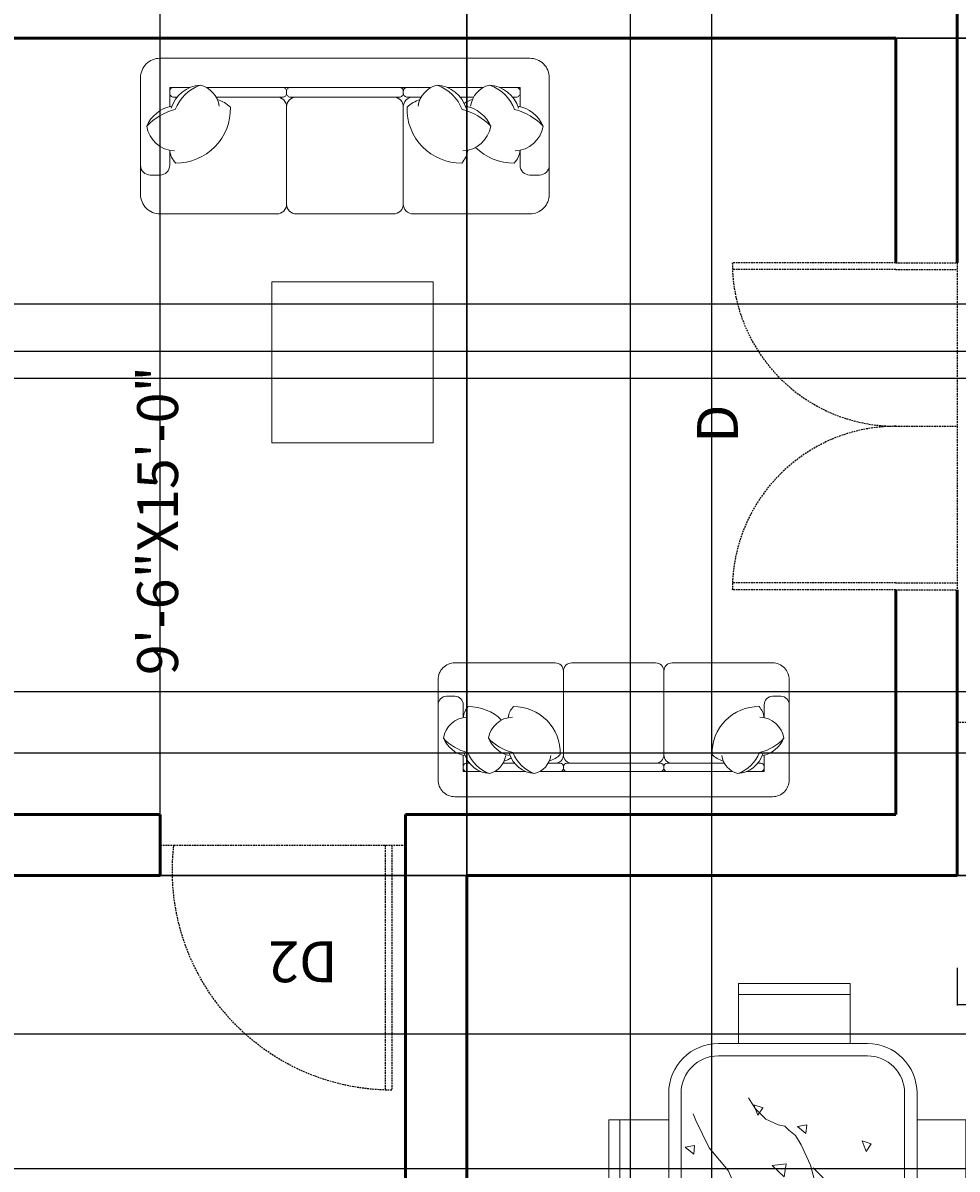
# Model space of a CAD drawing. Units: inches. Extents: x 3 to 576, y -689 to 51.
# Tile 8 of 21: x 199 to 336, y -429 to -261. Entities that reach past the tile are written whole.
import ezdxf

# ---------------------------------------------------------------- set-up
doc = ezdxf.new("R2010")
doc.units = ezdxf.units.IN
doc.header["$MEASUREMENT"] = 0
doc.linetypes.add('DASHED2', pattern=[0.375, 0.25, -0.125])
for name, color, linetype, lineweight in [('A-ANNO-DIMS', 2, 'Continuous', 18), ('A-ANNO-TEXT', 3, 'Continuous', 18), ('A-AREA-IDEN', 7, 'Continuous', 18), ('A-DOOR', 4, 'DASHED2', 25), ('A-FURN', 8, 'Continuous', 18), ('A-WALL', 7, 'Continuous', 50)]:
    doc.layers.add(name, color=color, linetype=linetype, lineweight=lineweight)
doc.styles.get("Standard").update_dxf_attribs({"font": 'arial.ttf'})
doc.dimstyles.get("Standard").update_dxf_attribs({"dimtxt": 0.18, "dimasz": 0.18, "dimexe": 0.18, "dimexo": 0.0625, "dimgap": 0.09, "dimtad": 0, "dimtih": 1, "dimtoh": 1, "dimdec": 0, "dimzin": 0, "dimdsep": 46, "dimlunit": 3, "dimtxsty": 'Standard', "dimcen": 0.09, "dimadec": 0, "dimazin": 0, "dimtfac": 1, "dimtdec": 0, "dimtofl": 0, "dimtmove": 0, "dimatfit": 3, "dimfxl": 1, "dimtolj": 1, "dimtzin": 0, "dimarcsym": 0})

# ---------------------------------------------------------------- blocks, each defined once
blk = doc.blocks.new('DINING-SET-6')
for p, q in [((35.44, 83.21), (19.03, 83.21)), ((19.03, 83.21), (19.03, 74.43)), ((35.44, 74.43), (35.44, 83.21)), ((19.03, 81.61), (35.44, 81.61)), ((37.96, 74.43), (16.08, 74.43)), ((16.08, 72.6), (37.96, 72.6)), ((8.79, 67.13), (8.79, 16.08)), ((10.61, 16.08), (10.61, 67.13)), ((20.49, 66.46), (21.48, 64.87)), ((43.43, 67.13), (43.43, 16.08)), ((45.25, 16.08), (45.25, 67.13)), ((12.38, 64.08), (12.77, 63.09)), ((21.9, 63.9), (21.31, 65.43)), ((22.64, 64.98), (21.31, 65.43)), ((21.48, 64.87), (23.07, 63.29)), ((21.9, 63.9), (22.63, 64.98)), ((0, 46.82), (0, 63.23)), ((0, 63.23), (8.79, 63.23)), ((1.6, 63.23), (1.6, 46.82)), ((12.77, 63.09), (14.75, 59.12)), ((23.07, 63.29), (24.85, 62.49)), ((24.85, 62.49), (25.84, 62.3)), ((25.84, 62.3), (26.44, 61.7)), ((29.06, 62.49), (27.69, 62.24)), ((28.94, 61.18), (29.06, 62.49)), ((54.04, 63.23), (45.25, 63.23)), ((52.44, 63.23), (52.44, 46.82)), ((54.04, 46.82), (54.04, 63.23)), ((26.44, 61.7), (27.43, 60.91)), ((27.43, 60.91), (28.22, 59.52)), ((28.94, 61.18), (27.69, 62.24)), ((12.6, 59.46), (11.23, 59.2)), ((12.49, 58.15), (11.23, 59.2)), ((12.49, 58.15), (12.6, 59.46)), ((14.75, 59.12), (17.52, 55.75)), ((28.22, 59.52), (29.6, 56.55)), ((38.5, 59.66), (37.18, 60.1)), ((37.77, 58.57), (37.18, 60.1)), ((37.77, 58.57), (38.5, 59.66)), ((17.52, 55.75), (18.51, 53.57)), ((26.06, 56.77), (23.98, 56.52)), ((25.76, 54.82), (23.98, 56.52)), ((25.76, 54.82), (26.06, 56.77)), ((29.6, 56.55), (30.2, 54.36)), ((30, 56.15), (30.79, 55.36)), ((30.2, 54.36), (31.39, 52.78)), ((30.79, 55.36), (32.18, 53.97)), ((32.18, 53.97), (33.96, 53.37)), ((13.09, 50.84), (12.5, 52.37)), ((13.83, 51.93), (12.5, 52.37)), ((18.51, 53.57), (18.51, 49.01)), ((31.39, 52.78), (32.77, 51.19)), ((33.96, 53.37), (34.36, 53.18)), ((34.36, 53.18), (35.35, 49.61)), ((13.09, 50.84), (13.83, 51.92)), ((19.11, 51.19), (19.11, 50)), ((32.77, 51.19), (33.76, 50.4)), ((18.51, 49.01), (17.52, 46.63)), ((19.11, 50), (19.5, 47.82)), ((33.76, 50.4), (34.75, 46.83)), ((35.35, 49.61), (36.73, 48.22)), ((39.5, 47.23), (41.09, 49.61)), ((41.09, 49.61), (41.49, 50)), ((43.43, 49.7), (42.77, 49.58)), ((43.43, 49.03), (42.77, 49.58)), ((19.5, 47.82), (19.5, 36.32)), ((36.73, 48.22), (37.92, 47.62)), ((37.92, 47.62), (38.71, 47.62)), ((38.71, 47.62), (39.5, 47.23)), ((8.79, 46.82), (0, 46.82)), ((17.52, 46.63), (17.92, 44.25)), ((27.69, 46.8), (26.31, 46.55)), ((27.57, 45.49), (26.31, 46.55)), ((27.57, 45.49), (27.68, 46.8)), ((28.96, 45.51), (28.37, 47.05)), ((29.69, 46.6), (28.37, 47.05)), ((28.96, 45.51), (29.69, 46.6)), ((34.75, 46.83), (35.15, 44.25)), ((45.25, 46.82), (54.04, 46.82)), ((17.92, 44.25), (18.12, 43.46)), ((19.5, 44.06), (20.09, 43.66)), ((35.15, 44.25), (35.54, 43.06)), ((11.23, 43.76), (10.61, 43.65)), ((11.11, 42.46), (10.61, 42.88)), ((11.11, 42.46), (11.23, 43.76)), ((20.09, 43.66), (21.08, 43.07)), ((21.08, 43.07), (21.68, 42.27)), ((21.68, 42.27), (22.67, 41.88)), ((35.54, 43.06), (35.15, 41.68)), ((22.67, 41.88), (23.46, 41.68)), ((23.46, 41.68), (23.85, 41.68)), ((23.85, 41.68), (24.45, 41.48)), ((35.15, 41.68), (36.14, 40.29)), ((0, 22.39), (0, 38.8)), ((0, 38.8), (8.79, 38.8)), ((1.6, 38.8), (1.6, 22.39)), ((36.14, 40.29), (36.73, 37.12)), ((54.04, 38.8), (45.25, 38.8)), ((52.44, 38.8), (52.44, 22.39)), ((54.04, 22.39), (54.04, 38.8)), ((19.5, 36.32), (19.9, 35.93)), ((19.9, 35.93), (23.27, 33.35)), ((20.15, 32.45), (19.56, 33.99)), ((20.88, 33.54), (19.56, 33.99)), ((42.77, 34.14), (41.4, 33.89)), ((42.65, 32.83), (41.4, 33.89)), ((42.65, 32.83), (42.77, 34.14)), ((20.15, 32.45), (20.88, 33.54)), ((22.44, 33.42), (20.36, 33.17)), ((22.14, 31.47), (20.36, 33.17)), ((22.14, 31.47), (22.44, 33.42)), ((23.27, 33.35), (26.24, 31.57)), ((23.86, 32.95), (25.64, 32.95)), ((25.64, 32.95), (27.03, 32.16)), ((27.03, 32.16), (27.82, 31.37)), ((26.31, 31.11), (24.94, 30.85)), ((26.2, 29.8), (24.94, 30.85)), ((26.24, 31.57), (25.84, 28.59)), ((26.2, 29.8), (26.31, 31.11)), ((27.82, 31.37), (28.81, 30.57)), ((36.01, 27.13), (35.43, 28.66)), ((36.75, 28.22), (35.43, 28.66)), ((25.84, 28.59), (25.84, 28)), ((36.01, 27.13), (36.75, 28.22)), ((40.69, 28), (38.9, 24.23)), ((38.9, 24.23), (38.9, 23.44)), ((8.79, 22.39), (0, 22.39)), ((38.9, 23.44), (39.3, 22.45)), ((39.3, 22.45), (38.9, 20.86)), ((45.25, 22.39), (54.04, 22.39)), ((11.34, 19.39), (10.75, 20.93)), ((12.07, 20.48), (10.75, 20.93)), ((11.34, 19.39), (12.07, 20.48)), ((30.99, 19.67), (29.8, 20.27)), ((38.9, 20.86), (37.72, 19.87)), ((31.78, 16.89), (30.99, 19.67)), ((37.72, 19.87), (37.52, 18.09)), ((32.18, 16.5), (31.78, 16.89)), ((37.52, 18.09), (36.92, 16.1)), ((41.28, 17.14), (40.02, 18.2)), ((41.4, 18.45), (40.03, 18.2)), ((41.28, 17.14), (41.4, 18.45)), ((24.94, 15.41), (23.57, 15.16)), ((24.82, 14.11), (23.57, 15.16)), ((24.82, 14.11), (24.94, 15.41)), ((27.21, 14.07), (26.62, 15.6)), ((27.94, 15.16), (26.62, 15.6)), ((27.21, 14.07), (27.94, 15.16)), ((32.57, 12.93), (32.18, 16.5)), ((36.92, 16.1), (36.13, 15.11)), ((36.13, 15.11), (35.74, 14.52)), ((32.57, 12.53), (32.57, 12.93)), ((35.15, 11.94), (32.57, 12.53)), ((36.14, 11.15), (35.15, 11.94)), ((42.34, 12.8), (41.67, 12.72)), ((42.01, 12.4), (41.67, 12.72)), ((37.96, 10.61), (16.08, 10.61)), ((37.13, 10.75), (36.14, 11.15)), ((16.08, 8.79), (37.96, 8.79)), ((19.03, 8.79), (19.03, 0)), ((35.44, 0), (35.44, 8.79)), ((35.44, 1.6), (19.03, 1.6)), ((19.03, 0), (35.44, 0))]:
    blk.add_line(p, q)
for centre, radius, start, end in [((16.08, 67.13), 7.29, 90, 180), ((37.96, 67.13), 7.29, 0, 90), ((16.08, 67.13), 5.47, 90, 180), ((37.96, 67.13), 5.47, 0, 90), ((16.08, 16.08), 7.29, 180, 270), ((16.08, 16.08), 5.47, 180, 270), ((37.96, 16.08), 5.47, 270, 0), ((37.96, 16.08), 7.29, 270, 0)]:
    blk.add_arc(centre, radius, start, end)
blk = doc.blocks.new('DOOR-900')
for p, q in [((34, 36), (0, 36)), ((2, 36), (2, 0)), ((36, 36), (34, 36))]:
    blk.add_line(p, q)
blk.add_arc((2, 32.22), 32.22, 270, 6.7329)
blk = doc.blocks.new('*D21')
at = {"layer": 'A-ANNO-DIMS', "color": 0, "lineweight": -2, "transparency": 16777216}
for p, q in [((336.29, -399.87), (336.29, -405.39)), ((372.29, -399.87), (372.29, -405.39)), ((336.47, -405.21), (353.05, -405.21)), ((372.11, -405.21), (355.54, -405.21))]:
    blk.add_line(p, q, dxfattribs=at)
at = {"layer": 'A-ANNO-DIMS', "color": 0, "transparency": 16777216}
for points in [[(336.47, -405.18), (336.47, -405.24), (336.29, -405.21)], [(372.11, -405.18), (372.11, -405.24), (372.29, -405.21)]]:
    blk.add_solid(points, dxfattribs=at)
at = {"layer": 'Defpoints', "color": 0, "transparency": 16777216}
for p in [(336.29, -399.81), (372.29, -399.81), (372.29, -405.21)]:
    blk.add_point(p, dxfattribs=at)
at = {"layer": 'A-ANNO-DIMS', "color": 0, "transparency": 16777216, "insert": (354.29, -405.21), "char_height": 0.18, "attachment_point": 5}
blk.add_mtext('\\A1;DOOR D1 3\'-0" TYP.', dxfattribs=at)
blk = doc.blocks.new('*D63')
at = {"layer": 'A-ANNO-DIMS', "color": 0, "lineweight": -2, "transparency": 16777216}
for p, q in [((47.36, -263.31), (575.92, -263.31)), ((575.74, -263.49), (575.74, -282.63)), ((575.74, -302.13), (575.74, -282.99)), ((47.36, -302.31), (575.92, -302.31))]:
    blk.add_line(p, q, dxfattribs=at)
at = {"layer": 'A-ANNO-DIMS', "color": 0, "transparency": 16777216}
for points in [[(575.71, -263.49), (575.77, -263.49), (575.74, -263.31)], [(575.71, -302.13), (575.77, -302.13), (575.74, -302.31)]]:
    blk.add_solid(points, dxfattribs=at)
at = {"layer": 'Defpoints', "color": 0, "transparency": 16777216}
for p in [(47.29, -263.31), (47.29, -302.31), (575.74, -302.31)]:
    blk.add_point(p, dxfattribs=at)
at = {"layer": 'A-ANNO-DIMS', "color": 0, "transparency": 16777216, "insert": (575.74, -282.81), "char_height": 0.18, "attachment_point": 5}
blk.add_mtext('\\A1;3\'-3"', dxfattribs=at)
blk = doc.blocks.new('*D68')
at = {"layer": 'A-ANNO-DIMS', "color": 0, "lineweight": -2, "transparency": 16777216}
for p, q in [((531.23, -254.31), (2.66, -254.31)), ((2.84, -254.49), (2.84, -258.63)), ((2.84, -263.13), (2.84, -258.99)), ((531.23, -263.31), (2.66, -263.31))]:
    blk.add_line(p, q, dxfattribs=at)
at = {"layer": 'A-ANNO-DIMS', "color": 0, "transparency": 16777216}
for points in [[(2.81, -254.49), (2.87, -254.49), (2.84, -254.31)], [(2.81, -263.13), (2.87, -263.13), (2.84, -263.31)]]:
    blk.add_solid(points, dxfattribs=at)
at = {"layer": 'Defpoints', "color": 0, "transparency": 16777216}
for p in [(531.29, -254.31), (2.84, -263.31), (531.29, -263.31)]:
    blk.add_point(p, dxfattribs=at)
at = {"layer": 'A-ANNO-DIMS', "color": 0, "transparency": 16777216, "insert": (2.84, -258.81), "char_height": 0.18, "attachment_point": 5}
blk.add_mtext('\\A1;0\'-9"', dxfattribs=at)
blk = doc.blocks.new('*D69')
at = {"layer": 'A-ANNO-DIMS', "color": 0, "lineweight": -2, "transparency": 16777216}
for p, q in [((531.23, -263.31), (2.66, -263.31)), ((2.84, -263.49), (2.84, -311.13)), ((2.84, -359.13), (2.84, -311.49)), ((531.23, -359.31), (2.66, -359.31))]:
    blk.add_line(p, q, dxfattribs=at)
at = {"layer": 'A-ANNO-DIMS', "color": 0, "transparency": 16777216}
for points in [[(2.81, -263.49), (2.87, -263.49), (2.84, -263.31)], [(2.81, -359.13), (2.87, -359.13), (2.84, -359.31)]]:
    blk.add_solid(points, dxfattribs=at)
at = {"layer": 'Defpoints', "color": 0, "transparency": 16777216}
for p in [(531.29, -263.31), (2.84, -359.31), (531.29, -359.31)]:
    blk.add_point(p, dxfattribs=at)
at = {"layer": 'A-ANNO-DIMS', "color": 0, "transparency": 16777216, "insert": (2.84, -311.31), "char_height": 0.18, "attachment_point": 5}
blk.add_mtext('\\A1;8\'-0"', dxfattribs=at)
blk = doc.blocks.new('*D70')
at = {"layer": 'A-ANNO-DIMS', "color": 0, "lineweight": -2, "transparency": 16777216}
for p, q in [((531.23, -359.31), (2.66, -359.31)), ((2.84, -359.49), (2.84, -363.63)), ((2.84, -368.13), (2.84, -363.99)), ((531.23, -368.31), (2.66, -368.31))]:
    blk.add_line(p, q, dxfattribs=at)
at = {"layer": 'A-ANNO-DIMS', "color": 0, "transparency": 16777216}
for points in [[(2.81, -359.49), (2.87, -359.49), (2.84, -359.31)], [(2.81, -368.13), (2.87, -368.13), (2.84, -368.31)]]:
    blk.add_solid(points, dxfattribs=at)
at = {"layer": 'Defpoints', "color": 0, "transparency": 16777216}
for p in [(531.29, -359.31), (2.84, -368.31), (531.29, -368.31)]:
    blk.add_point(p, dxfattribs=at)
at = {"layer": 'A-ANNO-DIMS', "color": 0, "transparency": 16777216, "insert": (2.84, -363.81), "char_height": 0.18, "attachment_point": 5}
blk.add_mtext('\\A1;0\'-9"', dxfattribs=at)
blk = doc.blocks.new('*D71')
at = {"layer": 'A-ANNO-DIMS', "color": 0, "lineweight": -2, "transparency": 16777216}
for p, q in [((531.23, -368.31), (2.66, -368.31)), ((2.84, -368.49), (2.84, -404.13)), ((2.84, -440.13), (2.84, -404.49)), ((531.23, -440.31), (2.66, -440.31))]:
    blk.add_line(p, q, dxfattribs=at)
at = {"layer": 'A-ANNO-DIMS', "color": 0, "transparency": 16777216}
for points in [[(2.81, -368.49), (2.87, -368.49), (2.84, -368.31)], [(2.81, -440.13), (2.87, -440.13), (2.84, -440.31)]]:
    blk.add_solid(points, dxfattribs=at)
at = {"layer": 'Defpoints', "color": 0, "transparency": 16777216}
for p in [(531.29, -368.31), (2.84, -440.31), (531.29, -440.31)]:
    blk.add_point(p, dxfattribs=at)
at = {"layer": 'A-ANNO-DIMS', "color": 0, "transparency": 16777216, "insert": (2.84, -404.31), "char_height": 0.18, "attachment_point": 5}
blk.add_mtext('\\A1;6\'-0"', dxfattribs=at)
blk = doc.blocks.new('*D84')
at = {"layer": 'A-ANNO-DIMS', "color": 0, "lineweight": -2, "transparency": 16777216}
for p, q in [((385.3, -263.31), (2.66, -263.31)), ((2.84, -263.49), (2.84, -286.13)), ((2.84, -309.13), (2.84, -286.49)), ((385.3, -309.31), (2.66, -309.31))]:
    blk.add_line(p, q, dxfattribs=at)
at = {"layer": 'A-ANNO-DIMS', "color": 0, "transparency": 16777216}
for points in [[(2.81, -263.49), (2.87, -263.49), (2.84, -263.31)], [(2.81, -309.13), (2.87, -309.13), (2.84, -309.31)]]:
    blk.add_solid(points, dxfattribs=at)
at = {"layer": 'Defpoints', "color": 0, "transparency": 16777216}
for p in [(385.37, -263.31), (2.84, -309.31), (385.37, -309.31)]:
    blk.add_point(p, dxfattribs=at)
at = {"layer": 'A-ANNO-DIMS', "color": 0, "transparency": 16777216, "insert": (2.84, -286.31), "char_height": 0.18, "attachment_point": 5}
blk.add_mtext('\\A1;3\'-10"', dxfattribs=at)
blk = doc.blocks.new('*D85')
at = {"layer": 'A-ANNO-DIMS', "color": 0, "lineweight": -2, "transparency": 16777216}
for p, q in [((385.3, -313.31), (2.66, -313.31)), ((2.84, -313.49), (2.84, -336.13)), ((2.84, -359.13), (2.84, -336.49)), ((385.3, -359.31), (2.66, -359.31))]:
    blk.add_line(p, q, dxfattribs=at)
at = {"layer": 'A-ANNO-DIMS', "color": 0, "transparency": 16777216}
for points in [[(2.81, -313.49), (2.87, -313.49), (2.84, -313.31)], [(2.81, -359.13), (2.87, -359.13), (2.84, -359.31)]]:
    blk.add_solid(points, dxfattribs=at)
at = {"layer": 'Defpoints', "color": 0, "transparency": 16777216}
for p in [(385.37, -313.31), (2.84, -359.31), (385.37, -359.31)]:
    blk.add_point(p, dxfattribs=at)
at = {"layer": 'A-ANNO-DIMS', "color": 0, "transparency": 16777216, "insert": (2.84, -336.31), "char_height": 0.18, "attachment_point": 5}
blk.add_mtext('\\A1;3\'-10"', dxfattribs=at)
blk = doc.blocks.new('*D91')
at = {"layer": 'A-ANNO-DIMS', "color": 0, "lineweight": -2, "transparency": 16777216}
for p, q in [((181.1, -386.31), (575.92, -386.31)), ((575.74, -386.49), (575.74, -397.75)), ((575.74, -409.38), (575.74, -398.11)), ((181.1, -409.56), (575.92, -409.56))]:
    blk.add_line(p, q, dxfattribs=at)
at = {"layer": 'A-ANNO-DIMS', "color": 0, "transparency": 16777216}
for points in [[(575.71, -386.49), (575.77, -386.49), (575.74, -386.31)], [(575.71, -409.38), (575.77, -409.38), (575.74, -409.56)]]:
    blk.add_solid(points, dxfattribs=at)
at = {"layer": 'Defpoints', "color": 0, "transparency": 16777216}
for p in [(181.04, -386.31), (181.04, -409.56), (575.74, -409.56)]:
    blk.add_point(p, dxfattribs=at)
at = {"layer": 'A-ANNO-DIMS', "color": 0, "transparency": 16777216, "insert": (575.74, -397.93), "char_height": 0.18, "attachment_point": 5}
blk.add_mtext('\\A1;1\'-11"', dxfattribs=at)
blk = doc.blocks.new('*D106')
at = {"layer": 'A-ANNO-DIMS', "color": 0, "lineweight": -2, "transparency": 16777216}
for p, q in [((111.36, -386.31), (575.92, -386.31)), ((575.74, -386.49), (575.74, -407.63)), ((575.74, -429.13), (575.74, -407.99)), ((111.36, -429.31), (575.92, -429.31))]:
    blk.add_line(p, q, dxfattribs=at)
at = {"layer": 'A-ANNO-DIMS', "color": 0, "transparency": 16777216}
for points in [[(575.71, -386.49), (575.77, -386.49), (575.74, -386.31)], [(575.71, -429.13), (575.77, -429.13), (575.74, -429.31)]]:
    blk.add_solid(points, dxfattribs=at)
at = {"layer": 'Defpoints', "color": 0, "transparency": 16777216}
for p in [(111.29, -386.31), (111.29, -429.31), (575.74, -429.31)]:
    blk.add_point(p, dxfattribs=at)
at = {"layer": 'A-ANNO-DIMS', "color": 0, "transparency": 16777216, "insert": (575.74, -407.81), "char_height": 0.18, "attachment_point": 5}
blk.add_mtext('\\A1;3\'-7"', dxfattribs=at)
blk = doc.blocks.new('*D114')
at = {"layer": 'A-ANNO-DIMS', "color": 0, "lineweight": -2, "transparency": 16777216}
for p, q in [((147.29, -377.25), (147.29, 51.32)), ((147.47, 51.14), (182.96, 51.14)), ((219.11, 51.14), (183.62, 51.14)), ((219.29, -377.25), (219.29, 51.32))]:
    blk.add_line(p, q, dxfattribs=at)
at = {"layer": 'A-ANNO-DIMS', "color": 0, "transparency": 16777216}
for points in [[(147.47, 51.17), (147.47, 51.11), (147.29, 51.14)], [(219.11, 51.17), (219.11, 51.11), (219.29, 51.14)]]:
    blk.add_solid(points, dxfattribs=at)
at = {"layer": 'Defpoints', "color": 0, "transparency": 16777216}
for p in [(219.29, 51.14), (147.29, -377.31), (219.29, -377.31)]:
    blk.add_point(p, dxfattribs=at)
at = {"layer": 'A-ANNO-DIMS', "color": 0, "transparency": 16777216, "insert": (183.29, 51.14), "char_height": 0.18, "attachment_point": 5}
blk.add_mtext('\\A1;6\'-0"', dxfattribs=at)
blk = doc.blocks.new('*D115')
at = {"layer": 'A-ANNO-DIMS', "color": 0, "lineweight": -2, "transparency": 16777216}
for p, q in [((264.29, -134.37), (264.29, -688.94)), ((288.29, -134.37), (288.29, -688.94)), ((264.47, -688.76), (275.96, -688.76)), ((288.11, -688.76), (276.62, -688.76))]:
    blk.add_line(p, q, dxfattribs=at)
at = {"layer": 'A-ANNO-DIMS', "color": 0, "transparency": 16777216}
for points in [[(264.47, -688.73), (264.47, -688.79), (264.29, -688.76)], [(288.11, -688.73), (288.11, -688.79), (288.29, -688.76)]]:
    blk.add_solid(points, dxfattribs=at)
at = {"layer": 'Defpoints', "color": 0, "transparency": 16777216}
for p in [(264.29, -134.31), (288.29, -134.31), (288.29, -688.76)]:
    blk.add_point(p, dxfattribs=at)
at = {"layer": 'A-ANNO-DIMS', "color": 0, "transparency": 16777216, "insert": (276.29, -688.76), "char_height": 0.18, "attachment_point": 5}
blk.add_mtext('\\A1;2\'-0"', dxfattribs=at)
blk = doc.blocks.new('*D117')
at = {"layer": 'A-ANNO-DIMS', "color": 0, "lineweight": -2, "transparency": 16777216}
for p, q in [((264.29, -506.25), (264.29, 51.32)), ((264.47, 51.14), (281.96, 51.14)), ((300.11, 51.14), (282.62, 51.14)), ((300.29, -506.25), (300.29, 51.32))]:
    blk.add_line(p, q, dxfattribs=at)
at = {"layer": 'A-ANNO-DIMS', "color": 0, "transparency": 16777216}
for points in [[(264.47, 51.17), (264.47, 51.11), (264.29, 51.14)], [(300.11, 51.17), (300.11, 51.11), (300.29, 51.14)]]:
    blk.add_solid(points, dxfattribs=at)
at = {"layer": 'Defpoints', "color": 0, "transparency": 16777216}
for p in [(300.29, 51.14), (264.29, -506.31), (300.29, -506.31)]:
    blk.add_point(p, dxfattribs=at)
at = {"layer": 'A-ANNO-DIMS', "color": 0, "transparency": 16777216, "insert": (282.29, 51.14), "char_height": 0.18, "attachment_point": 5}
blk.add_mtext('\\A1;3\'-0"', dxfattribs=at)
blk = doc.blocks.new('*D125')
at = {"layer": 'A-ANNO-DIMS', "color": 0, "lineweight": -2, "transparency": 16777216}
for p, q in [((531.23, -368.31), (2.66, -368.31)), ((2.84, -368.49), (2.84, -377.13)), ((2.84, -386.13), (2.84, -377.49)), ((512.45, -386.31), (2.66, -386.31))]:
    blk.add_line(p, q, dxfattribs=at)
at = {"layer": 'A-ANNO-DIMS', "color": 0, "transparency": 16777216}
for points in [[(2.81, -368.49), (2.87, -368.49), (2.84, -368.31)], [(2.81, -386.13), (2.87, -386.13), (2.84, -386.31)]]:
    blk.add_solid(points, dxfattribs=at)
at = {"layer": 'Defpoints', "color": 0, "transparency": 16777216}
for p in [(531.29, -368.31), (2.84, -386.31), (512.51, -386.31)]:
    blk.add_point(p, dxfattribs=at)
at = {"layer": 'A-ANNO-DIMS', "color": 0, "transparency": 16777216, "insert": (2.84, -377.31), "char_height": 0.18, "attachment_point": 5}
blk.add_mtext('\\A1;1\'-6"', dxfattribs=at)

msp = doc.modelspace()

# ---------------------------------------------------------------- linework, layer by layer
at = {"layer": 'A-DOOR'}
for p, q in [((327.29, -296.31), (303.29, -296.31)), ((327.29, -297.31), (303.29, -297.31)), ((327.29, -296.31), (336.29, -296.31)), ((327.29, -297.31), (336.29, -297.31)), ((336.29, -296.31), (336.29, -344.31)), ((327.29, -320.31), (336.29, -320.31)), ((327.29, -343.31), (303.29, -343.31)), ((327.29, -343.31), (336.29, -343.31)), ((327.29, -344.31), (303.29, -344.31)), ((327.29, -344.31), (336.29, -344.31)), ((252.29, -381.81), (252.29, -417.81))]:
    msp.add_line(p, q, dxfattribs=at)
for centre, start, end in [((327.29, -296.31), 180, 270), ((327.29, -344.31), 90, 180)]:
    msp.add_arc(centre, 24, start, end, dxfattribs=at)
at = {"layer": 'A-FURN', "ltscale": 0.03}
for points in [[(216.39, -286.26, 0.414214), (219.25, -289.12), (236.4, -289.12, 0.414214), (237.83, -287.69, 0.414214), (239.26, -289.12), (253.55, -289.12, 0.414214), (254.98, -287.69, 0.414214), (256.41, -289.12), (273.56, -289.12, 0.414214), (276.41, -286.26), (276.41, -269.11, 0.414214), (273.56, -266.26), (219.25, -266.26, 0.414214), (216.39, -269.11)], [(311.65, -357.52, 0.414214), (309.2, -355.06), (294.46, -355.06, 0.414214), (293.24, -356.29, 0.414214), (292.01, -355.06), (279.73, -355.06, 0.414214), (278.5, -356.29, 0.414214), (277.27, -355.06), (262.54, -355.06, 0.414214), (260.08, -357.52), (260.08, -372.25, 0.414214), (262.54, -374.71), (309.2, -374.71, 0.414214), (311.65, -372.25)]]:
    msp.add_lwpolyline(points, format="xyb", close=True, dxfattribs=at)
at = {"layer": 'A-FURN'}
for points in [[(217.3, -276.25, -0.14773), (221.48, -273.79, -0.213343), (225.16, -270.19, -0.178662)], [(221.77, -271.97), (221.25, -271.97, -0.414214), (220.68, -271.4), (220.68, -271.12, -0.414214), (221.25, -270.54)], [(220.9, -273.6, -0.306663), (225.16, -270.19, -0.30633), (227.95, -273.3, 0.872847)], [(221.25, -270.54), (223.68, -270.54, -0.414214)], [(226.06, -270.54), (237.25, -270.54, -0.414214), (237.83, -271.12), (237.83, -271.4, -0.414214), (237.25, -271.97), (227.5, -271.97, -0.414214)], [(259.04, -270.54), (255.55, -270.54, 0.414214), (254.98, -271.12), (254.98, -271.4, 0.414214), (255.55, -271.97), (257.6, -271.97, 0.414214)], [(264.21, -273.6, 0.306663), (259.94, -270.19, 0.30633), (257.16, -273.3, -0.872847)], [(267.81, -276.25, 0.14773), (263.63, -273.79, 0.213343), (259.94, -270.19, 0.178662)], [(266.74, -270.54), (261.42, -270.54, 0.414214)], [(271.91, -273.6, 0.306663), (267.64, -270.19, 0.30633), (264.86, -273.3, -0.872847)], [(275.51, -276.25, 0.14773), (271.33, -273.79, 0.213343), (267.64, -270.19, 0.178662)], [(269.12, -270.54), (272.13, -270.54), (272.13, -273.35, 0.414214)], [(271.56, -270.54), (269.12, -270.54, 0.414214)], [(271.04, -271.97), (271.56, -271.97, 0.414214), (272.13, -271.4), (272.13, -271.12, 0.414214), (271.56, -270.54)], [(220.67, -279.76, 0.165541), (221.56, -281.65, 0.425989), (229.58, -273.46, 0.121523), (227.68, -272.33, -7.115464)], [(236.4, -271.97, -0.414214), (237.83, -273.4), (237.83, -287.69, -0.414214)], [(239.26, -271.97, 0.414214), (237.83, -273.4)], [(253.55, -271.97, -0.414214), (254.98, -273.4)], [(256.41, -271.97, 0.414214), (254.98, -273.4), (254.98, -287.69, 0.414214)], [(264.43, -279.76, -0.165541), (263.55, -281.65, -0.425989), (255.52, -273.46, -0.121523), (257.43, -272.33, 7.115464)], [(263.34, -271.97), (265.3, -271.97, 0.414214)], [(263.93, -272.89, -0.071865), (265.12, -272.33, 7.115464)], [(221.39, -279.85, -0.356772), (217.3, -276.25, -0.249542), (221.01, -273.28, 9.61688)], [(263.71, -279.85, 0.356772), (267.81, -276.25, 0.249542), (264.1, -273.28, -9.61688)], [(271.41, -279.85, 0.356772), (275.51, -276.25, 0.249542), (271.79, -273.28, -9.61688)], [(272.13, -279.76, -0.165541), (271.25, -281.65, -0.200231), (265.57, -279.35, -0.121523)], [(216.39, -281.98, 0.414214), (217.82, -283.41), (219.25, -283.41, 0.414214), (220.68, -281.98), (220.68, -279.76)], [(272.13, -279.76), (272.13, -281.98, 0.414214), (273.56, -283.41), (274.99, -283.41, 0.414214), (276.41, -281.98)], [(277.27, -369.8, 0.414214), (278.5, -368.57), (278.5, -356.29, 0.414214)], [(294.46, -369.8, -0.414214), (293.24, -368.57), (293.24, -356.29, -0.414214)], [(263.77, -363.1), (263.77, -361.2, 0.414214), (262.54, -359.97), (261.31, -359.97, 0.414214), (260.08, -361.2)], [(311.65, -361.2, 0.414214), (310.43, -359.97), (309.2, -359.97, 0.414214), (307.97, -361.2), (307.97, -363.1)], [(263.76, -363.11, -0.165541), (264.52, -361.48, -0.200231), (269.4, -363.46, -0.121523)], [(270.38, -363.11, -0.165541), (271.14, -361.48, -0.425989), (278.03, -368.52, -0.121523), (276.4, -369.49, 7.115464)], [(307.97, -363.11, 0.165541), (307.21, -361.48, 0.425989), (300.32, -368.52, 0.121523), (301.95, -369.49, -7.115464)], [(264.38, -363.03, 0.356772), (260.86, -366.13, 0.249542), (264.05, -368.68, -9.61688)], [(271, -363.03, 0.356772), (267.48, -366.13, 0.249542), (270.67, -368.68, -9.61688)], [(307.35, -363.03, -0.356772), (310.87, -366.13, -0.249542), (307.68, -368.68, 9.61688)], [(260.86, -366.13, 0.14773), (264.45, -368.24, 0.213343), (267.62, -371.33, 0.178662)], [(267.48, -366.13, 0.14773), (271.07, -368.24, 0.213343), (274.23, -371.33, 0.178662)], [(310.87, -366.13, -0.14773), (307.28, -368.24, -0.213343), (304.12, -371.33, -0.178662)], [(266.35, -371.03), (263.77, -371.03), (263.77, -368.61, 0.414214)], [(263.96, -368.4, 0.306663), (267.62, -371.33, 0.30633), (270.01, -368.66, -0.872847)], [(270.57, -368.4, 0.306663), (274.23, -371.33, 0.30633), (276.63, -368.66, -0.872847)], [(279.73, -369.8, -0.414214), (278.5, -368.57)], [(292.01, -369.8, 0.414214), (293.24, -368.57)], [(307.78, -368.4, -0.306663), (304.12, -371.33, -0.30633), (301.73, -368.66, 0.872847)], [(264.7, -369.8), (264.26, -369.8, 0.414214), (263.77, -370.29), (263.77, -370.53, 0.414214), (264.26, -371.03)], [(271.32, -369.8), (269.63, -369.8, 0.414214)], [(270.81, -369.01, -0.071865), (269.78, -369.49, 7.115464)], [(275.01, -371.03), (278.01, -371.03, 0.414214), (278.5, -370.53), (278.5, -370.29, 0.414214), (278.01, -369.8), (276.24, -369.8, 0.414214)], [(303.34, -371.03), (293.73, -371.03, -0.414214), (293.24, -370.53), (293.24, -370.29, -0.414214), (293.73, -369.8), (302.11, -369.8, -0.414214)], [(307.03, -369.8), (307.48, -369.8, -0.414214), (307.97, -370.29), (307.97, -370.53, -0.414214), (307.48, -371.03)], [(264.26, -371.03), (266.35, -371.03, 0.414214)], [(268.39, -371.03), (272.96, -371.03, 0.414214)], [(307.48, -371.03), (305.39, -371.03, -0.414214)]]:
    msp.add_lwpolyline(points, format="xyb", dxfattribs=at)
for points in [[(220.68, -273.35), (220.68, -270.54), (223.68, -270.54)], [(226.06, -270.54), (259.04, -270.54)], [(261.42, -270.54), (266.74, -270.54)], [(307.97, -368.61), (307.97, -371.03), (305.39, -371.03)], [(272.96, -371.03), (268.39, -371.03)], [(303.34, -371.03), (275.01, -371.03)]]:
    msp.add_lwpolyline(points, dxfattribs=at)
for points in [[(254.41, -270.54), (238.4, -270.54, 0.414214), (237.83, -271.12), (237.83, -271.4, 0.414214), (238.4, -271.97), (254.41, -271.97, 0.414214), (254.98, -271.4), (254.98, -271.12, 0.414214)], [(278.99, -371.03), (292.74, -371.03, 0.414214), (293.24, -370.53), (293.24, -370.29, 0.414214), (292.74, -369.8), (278.99, -369.8, 0.414214), (278.5, -370.29), (278.5, -370.53, 0.414214)]]:
    msp.add_lwpolyline(points, format="xyb", close=True, dxfattribs=at)
at = {"layer": 'A-FURN', "ltscale": 0.03}
msp.add_lwpolyline([(259.36, -299.09), (259.36, -322.76), (235.68, -322.76), (235.68, -299.09)], close=True, dxfattribs=at)
at = {"layer": 'A-WALL'}
for p, q in [((336.29, -254.31), (336.29, -263.31)), ((147.29, -263.31), (327.29, -263.31)), ((327.29, -263.31), (327.29, -296.31)), ((336.29, -263.31), (336.29, -296.31)), ((327.29, -344.31), (327.29, -377.31)), ((336.29, -344.31), (336.29, -386.31)), ((147.29, -377.31), (219.29, -377.31)), ((219.29, -386.31), (219.29, -377.31)), ((255.29, -386.31), (255.29, -377.31)), ((255.29, -377.31), (327.29, -377.31)), ((111.29, -386.31), (219.29, -386.31)), ((255.29, -386.31), (255.29, -506.31)), ((264.29, -386.31), (264.29, -506.31)), ((264.29, -386.31), (336.29, -386.31))]:
    msp.add_line(p, q, dxfattribs=at)

# ---------------------------------------------------------------- block references
at = {"layer": 'A-DOOR'}
msp.add_blockref('DOOR-900', (336.29, -399.81), dxfattribs=at)
at = {"layer": 'A-DOOR', "extrusion": (0, 0, -1), "zscale": -1}
msp.add_blockref('DOOR-900', (-255.29, -417.81), dxfattribs=at)
at = {"layer": 'A-FURN'}
msp.add_blockref('DINING-SET-6', (285.16, -485.38), dxfattribs=at)

# ---------------------------------------------------------------- texts
at = {"layer": 'A-ANNO-TEXT', "char_height": 6, "attachment_point": 1}
for s, insert, rotation in [('D', (298.11, -322.75), 90), ('D2', (245.32, -401.96), 180)]:
    msp.add_mtext(s, dxfattribs=dict(at, insert=insert, rotation=rotation))
at = {"layer": 'A-AREA-IDEN', "insert": (215.9, -356.86), "char_height": 6, "attachment_point": 1, "rotation": 90}
msp.add_mtext('9\'-6"X15\'-0"', dxfattribs=at)

# ---------------------------------------------------------------- dimensions: what is measured, and where the dimension line sits
at = {"layer": 'A-ANNO-DIMS'}
for base, p1, p2, picture, middle in [((219.29, 51.14), (147.29, -377.31), (219.29, -377.31), '*D114', (183.29, 51.14)), ((300.29, 51.14), (264.29, -506.31), (300.29, -506.31), '*D117', (282.29, 51.14)), ((288.29, -688.76), (264.29, -134.31), (288.29, -134.31), '*D115', (276.29, -688.76))]:
    dim = msp.add_linear_dim(base=base, p1=p1, p2=p2, dimstyle='Standard', override={"dimdec": 1, "dimlfac": 1, "dimrnd": 0, "dimzin": 1, "dimdsep": 46, "dimlunit": 4, "dimfrac": 2}, dxfattribs=at)
    dim.commit()
    dim.dimension.update_dxf_attribs({"geometry": picture, "text_midpoint": middle})
for base, p1, p2, picture, middle in [((2.84, -263.31), (531.29, -254.31), (531.29, -263.31), '*D68', (2.84, -258.81)), ((2.84, -309.31), (385.37, -263.31), (385.37, -309.31), '*D84', (2.84, -286.31)), ((2.84, -359.31), (531.29, -263.31), (531.29, -359.31), '*D69', (2.84, -311.31)), ((575.74, -302.31), (47.29, -263.31), (47.29, -302.31), '*D63', (575.74, -282.81)), ((2.84, -359.31), (385.37, -313.31), (385.37, -359.31), '*D85', (2.84, -336.31)), ((2.84, -368.31), (531.29, -359.31), (531.29, -368.31), '*D70', (2.84, -363.81)), ((2.84, -440.31), (531.29, -368.31), (531.29, -440.31), '*D71', (2.84, -404.31)), ((2.84, -386.31), (531.29, -368.31), (512.51, -386.31), '*D125', (2.84, -377.31)), ((575.74, -429.31), (111.29, -386.31), (111.29, -429.31), '*D106', (575.74, -407.81)), ((575.744, -409.5571), (181.036, -386.3097), (181.036, -409.5571), '*D91', (575.744, -397.9334))]:
    dim = msp.add_linear_dim(base=base, p1=p1, p2=p2, angle=90, dimstyle='Standard', override={"dimdec": 1, "dimlfac": 1, "dimrnd": 0, "dimzin": 1, "dimdsep": 46, "dimlunit": 4, "dimfrac": 2}, dxfattribs=at)
    dim.commit()
    dim.dimension.update_dxf_attribs({"geometry": picture, "text_midpoint": middle})
dim = msp.add_linear_dim(base=(372.29, -405.21), p1=(336.29, -399.81), p2=(372.29, -399.81), text='DOOR D1 <> TYP.', dimstyle='Standard', override={"dimdec": 1, "dimlfac": 1, "dimrnd": 0, "dimzin": 1, "dimdsep": 46, "dimlunit": 4, "dimfrac": 2}, dxfattribs=at)
dim.commit()
dim.dimension.update_dxf_attribs({"geometry": '*D21', "text_midpoint": (354.29, -405.21)})

doc.saveas('drawing.dxf')
